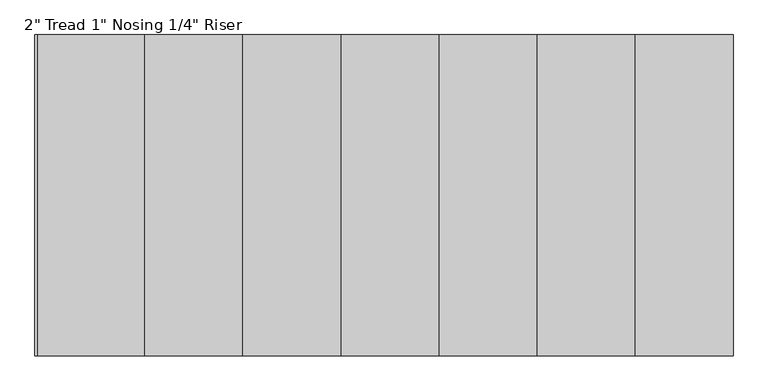
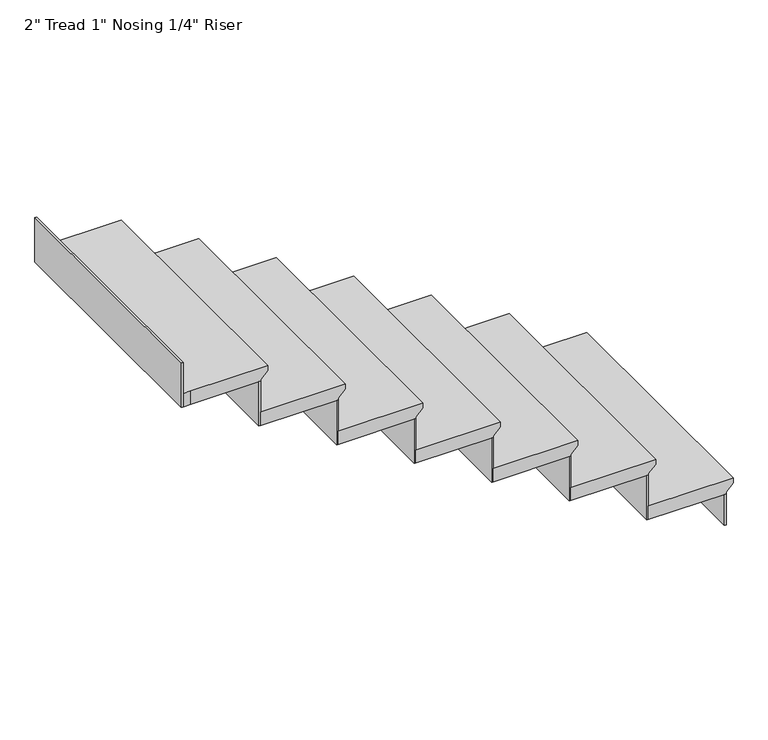
"""IFC4 building model written with IfcOpenShell, lengths in millimetres: stair flight geometry."""

from ifc_helpers import new_model, si_unit, origin, place, context, project, spatial, faceted_brep, source, transform, mapped, element, save


def stair_flight_155d8820(model_context):
    return source(origin(), model_context, "Body", "Brep", [
        faceted_brep([(-12620.1777023, 559.4679075, 455.0833333), (-12620.1777023, 559.4679075, 474.1333333), (-12620.1777023, -354.9320925, 474.1333333), (-12620.1777023, -354.9320925, 455.0833333), (-12645.5777023, 559.4679075, 429.6833333), (-12645.5777023, -354.9320925, 429.6833333), (-12924.9777023, 559.4679075, 474.1333333), (-12924.9777023, -354.9320925, 474.1333333), (-12645.5777023, -354.9320925, 423.3333333), (-12924.9777023, -354.9320925, 423.3333333), (-12924.9777023, 559.4679075, 423.3333333), (-12645.5777023, 559.4679075, 423.3333333)], [[[0, 1, 2, 3]], [[4, 0, 3, 5]], [[2, 1, 6, 7]], [[8, 9, 10, 11]], [[2, 7, 9, 8, 5, 3]], [[8, 11, 4, 5]], [[6, 1, 0, 4, 11, 10]], [[7, 6, 10, 9]]]),
        faceted_brep([(-12645.5777023, 559.4679075, 423.3333333), (-12645.5777023, 559.4679075, 304.8), (-12651.9277023, 559.4679075, 304.8), (-12651.9277023, 559.4679075, 423.3333333), (-12645.5777023, -354.9320925, 423.3333333), (-12651.9277023, -354.9320925, 423.3333333), (-12651.9277023, -354.9320925, 304.8), (-12645.5777023, -354.9320925, 304.8)], [[[0, 1, 2, 3]], [[4, 5, 6, 7]], [[1, 0, 4, 7]], [[2, 1, 7, 6]], [[3, 2, 6, 5]], [[0, 3, 5, 4]]]),
        faceted_brep([(-12924.9777023, 559.4679075, 592.6666667), (-12924.9777023, 559.4679075, 423.3333333), (-12931.3277023, 559.4679075, 423.3333333), (-12931.3277023, 559.4679075, 592.6666667), (-12924.9777023, -354.9320925, 592.6666667), (-12931.3277023, -354.9320925, 592.6666667), (-12931.3277023, -354.9320925, 423.3333333), (-12924.9777023, -354.9320925, 423.3333333)], [[[0, 1, 2, 3]], [[4, 5, 6, 7]], [[1, 0, 4, 7]], [[2, 1, 7, 6]], [[3, 2, 6, 5]], [[0, 3, 5, 4]]]),
        faceted_brep([(-12899.5777023, -354.9320925, 643.4666667), (-12899.5777023, 559.4679075, 643.4666667), (-13204.3777023, 559.4679075, 643.4666667), (-13204.3777023, -354.9320925, 643.4666667), (-12924.9777023, -354.9320925, 592.6666667), (-13204.3777023, -354.9320925, 592.6666667), (-13204.3777023, 559.4679075, 592.6666667), (-12924.9777023, 559.4679075, 592.6666667), (-12924.9777023, -354.9320925, 599.0166667), (-12899.5777023, -354.9320925, 624.4166667), (-12924.9777023, 559.4679075, 599.0166667), (-12899.5777023, 559.4679075, 624.4166667)], [[[0, 1, 2, 3]], [[4, 5, 6, 7]], [[0, 3, 5, 4, 8, 9]], [[4, 7, 10, 8]], [[2, 1, 11, 10, 7, 6]], [[3, 2, 6, 5]], [[11, 1, 0, 9]], [[10, 11, 9, 8]]]),
        faceted_brep([(-13204.3777023, 559.4679075, 762.0), (-13204.3777023, 559.4679075, 592.6666667), (-13210.7277023, 559.4679075, 592.6666667), (-13210.7277023, 559.4679075, 762.0), (-13204.3777023, -354.9320925, 762.0), (-13210.7277023, -354.9320925, 762.0), (-13210.7277023, -354.9320925, 592.6666667), (-13204.3777023, -354.9320925, 592.6666667)], [[[0, 1, 2, 3]], [[4, 5, 6, 7]], [[1, 0, 4, 7]], [[2, 1, 7, 6]], [[3, 2, 6, 5]], [[0, 3, 5, 4]]]),
        faceted_brep([(-13178.9777023, -354.9320925, 812.8), (-13178.9777023, 559.4679075, 812.8), (-13483.7777023, 559.4679075, 812.8), (-13483.7777023, -354.9320925, 812.8), (-13204.3777023, -354.9320925, 762.0), (-13483.7777023, -354.9320925, 762.0), (-13483.7777023, 559.4679075, 762.0), (-13204.3777023, 559.4679075, 762.0), (-13204.3777023, -354.9320925, 768.35), (-13178.9777023, -354.9320925, 793.75), (-13204.3777023, 559.4679075, 768.35), (-13178.9777023, 559.4679075, 793.75)], [[[0, 1, 2, 3]], [[4, 5, 6, 7]], [[0, 3, 5, 4, 8, 9]], [[4, 7, 10, 8]], [[2, 1, 11, 10, 7, 6]], [[3, 2, 6, 5]], [[11, 1, 0, 9]], [[10, 11, 9, 8]]]),
        faceted_brep([(-13483.7777023, 559.4679075, 931.3333333), (-13483.7777023, 559.4679075, 762.0), (-13490.1277023, 559.4679075, 762.0), (-13490.1277023, 559.4679075, 931.3333333), (-13483.7777023, -354.9320925, 931.3333333), (-13490.1277023, -354.9320925, 931.3333333), (-13490.1277023, -354.9320925, 762.0), (-13483.7777023, -354.9320925, 762.0)], [[[0, 1, 2, 3]], [[4, 5, 6, 7]], [[1, 0, 4, 7]], [[2, 1, 7, 6]], [[3, 2, 6, 5]], [[0, 3, 5, 4]]]),
        faceted_brep([(-13458.3777023, -354.9320925, 982.1333333), (-13458.3777023, 559.4679075, 982.1333333), (-13763.1777023, 559.4679075, 982.1333333), (-13763.1777023, -354.9320925, 982.1333333), (-13483.7777023, -354.9320925, 931.3333333), (-13763.1777023, -354.9320925, 931.3333333), (-13763.1777023, 559.4679075, 931.3333333), (-13483.7777023, 559.4679075, 931.3333333), (-13483.7777023, -354.9320925, 937.6833333), (-13458.3777023, -354.9320925, 963.0833333), (-13483.7777023, 559.4679075, 937.6833333), (-13458.3777023, 559.4679075, 963.0833333)], [[[0, 1, 2, 3]], [[4, 5, 6, 7]], [[0, 3, 5, 4, 8, 9]], [[4, 7, 10, 8]], [[2, 1, 11, 10, 7, 6]], [[3, 2, 6, 5]], [[11, 1, 0, 9]], [[10, 11, 9, 8]]]),
        faceted_brep([(-13763.1777023, 559.4679075, 1100.6666667), (-13763.1777023, 559.4679075, 931.3333333), (-13769.5277023, 559.4679075, 931.3333333), (-13769.5277023, 559.4679075, 1100.6666667), (-13763.1777023, -354.9320925, 1100.6666667), (-13769.5277023, -354.9320925, 1100.6666667), (-13769.5277023, -354.9320925, 931.3333333), (-13763.1777023, -354.9320925, 931.3333333)], [[[0, 1, 2, 3]], [[4, 5, 6, 7]], [[1, 0, 4, 7]], [[2, 1, 7, 6]], [[3, 2, 6, 5]], [[0, 3, 5, 4]]]),
        faceted_brep([(-13737.7777023, -354.9320925, 1151.4666667), (-13737.7777023, 559.4679075, 1151.4666667), (-14042.5777023, 559.4679075, 1151.4666667), (-14042.5777023, -354.9320925, 1151.4666667), (-13763.1777023, -354.9320925, 1100.6666667), (-14042.5777023, -354.9320925, 1100.6666667), (-14042.5777023, 559.4679075, 1100.6666667), (-13763.1777023, 559.4679075, 1100.6666667), (-13763.1777023, -354.9320925, 1107.0166667), (-13737.7777023, -354.9320925, 1132.4166667), (-13763.1777023, 559.4679075, 1107.0166667), (-13737.7777023, 559.4679075, 1132.4166667)], [[[0, 1, 2, 3]], [[4, 5, 6, 7]], [[0, 3, 5, 4, 8, 9]], [[4, 7, 10, 8]], [[2, 1, 11, 10, 7, 6]], [[3, 2, 6, 5]], [[11, 1, 0, 9]], [[10, 11, 9, 8]]]),
        faceted_brep([(-14042.5777023, 559.4679075, 1270.0), (-14042.5777023, 559.4679075, 1100.6666667), (-14048.9277023, 559.4679075, 1100.6666667), (-14048.9277023, 559.4679075, 1270.0), (-14042.5777023, -354.9320925, 1270.0), (-14048.9277023, -354.9320925, 1270.0), (-14048.9277023, -354.9320925, 1100.6666667), (-14042.5777023, -354.9320925, 1100.6666667)], [[[0, 1, 2, 3]], [[4, 5, 6, 7]], [[1, 0, 4, 7]], [[2, 1, 7, 6]], [[3, 2, 6, 5]], [[0, 3, 5, 4]]]),
        faceted_brep([(-14017.1777023, -354.9320925, 1320.8), (-14017.1777023, 559.4679075, 1320.8), (-14321.9777023, 559.4679075, 1320.8), (-14321.9777023, -354.9320925, 1320.8), (-14042.5777023, -354.9320925, 1270.0), (-14321.9777023, -354.9320925, 1270.0), (-14321.9777023, 559.4679075, 1270.0), (-14042.5777023, 559.4679075, 1270.0), (-14042.5777023, -354.9320925, 1276.35), (-14017.1777023, -354.9320925, 1301.75), (-14042.5777023, 559.4679075, 1276.35), (-14017.1777023, 559.4679075, 1301.75)], [[[0, 1, 2, 3]], [[4, 5, 6, 7]], [[0, 3, 5, 4, 8, 9]], [[4, 7, 10, 8]], [[2, 1, 11, 10, 7, 6]], [[3, 2, 6, 5]], [[11, 1, 0, 9]], [[10, 11, 9, 8]]]),
        faceted_brep([(-14601.3777023, 559.4679075, 1608.6666667), (-14601.3777023, 559.4679075, 1439.3333333), (-14607.7277023, 559.4679075, 1439.3333333), (-14607.7277023, 559.4679075, 1608.6666667), (-14601.3777023, -354.9320925, 1608.6666667), (-14607.7277023, -354.9320925, 1608.6666667), (-14607.7277023, -354.9320925, 1439.3333333), (-14601.3777023, -354.9320925, 1439.3333333)], [[[0, 1, 2, 3]], [[4, 5, 6, 7]], [[1, 0, 4, 7]], [[2, 1, 7, 6]], [[3, 2, 6, 5]], [[0, 3, 5, 4]]]),
        faceted_brep([(-14321.9777023, 559.4679075, 1439.3333333), (-14321.9777023, 559.4679075, 1270.0), (-14328.3277023, 559.4679075, 1270.0), (-14328.3277023, 559.4679075, 1439.3333333), (-14321.9777023, -354.9320925, 1439.3333333), (-14328.3277023, -354.9320925, 1439.3333333), (-14328.3277023, -354.9320925, 1270.0), (-14321.9777023, -354.9320925, 1270.0)], [[[0, 1, 2, 3]], [[4, 5, 6, 7]], [[1, 0, 4, 7]], [[2, 1, 7, 6]], [[3, 2, 6, 5]], [[0, 3, 5, 4]]]),
        faceted_brep([(-14601.3777023, -354.9320925, 1490.1333333), (-14575.9777023, -354.9320925, 1490.1333333), (-14296.5777023, -354.9320925, 1490.1333333), (-14296.5777023, 559.4679075, 1490.1333333), (-14601.3777023, 559.4679075, 1490.1333333), (-14575.9777023, -354.9320925, 1439.3333333), (-14601.3777023, -354.9320925, 1439.3333333), (-14601.3777023, 559.4679075, 1439.3333333), (-14321.9777023, 559.4679075, 1439.3333333), (-14321.9777023, -354.9320925, 1439.3333333), (-14321.9777023, -354.9320925, 1445.6833333), (-14296.5777023, -354.9320925, 1471.0833333), (-14321.9777023, 559.4679075, 1445.6833333), (-14296.5777023, 559.4679075, 1471.0833333)], [[[0, 1, 2, 3, 4]], [[5, 6, 7, 8, 9]], [[1, 0, 6, 5]], [[2, 1, 5, 9, 10, 11]], [[9, 8, 12, 10]], [[4, 3, 13, 12, 8, 7]], [[0, 4, 7, 6]], [[13, 3, 2, 11]], [[12, 13, 11, 10]]]),
    ])


if __name__ == "__main__":
    model = new_model("IFC4")
    model_context = context("Model", 3, world=origin())
    ifc_project = project(units=[si_unit("LENGTHUNIT", "METRE", prefix="MILLI")], contexts=[model_context])
    site = spatial("IfcSite", under=ifc_project)
    building = spatial("IfcBuilding", under=site)
    placement = place(None, origin())
    stair_flight_shape = stair_flight_155d8820(model_context)
    element("IfcStairFlight", 1, ObjectType="2\" Tread 1\" Nosing 1/4\" Riser", at=placement, inside=building, context=model_context, shape_type="MappedRepresentation", body=[
        mapped(stair_flight_shape, transform((0.0, 0.0, 0.0), x_axis=(1.0, 0.0, 0.0), y_axis=(0.0, 1.0, 0.0), z_axis=(0.0, 0.0, 1.0))),
    ])
    save(model, "model.ifc")
